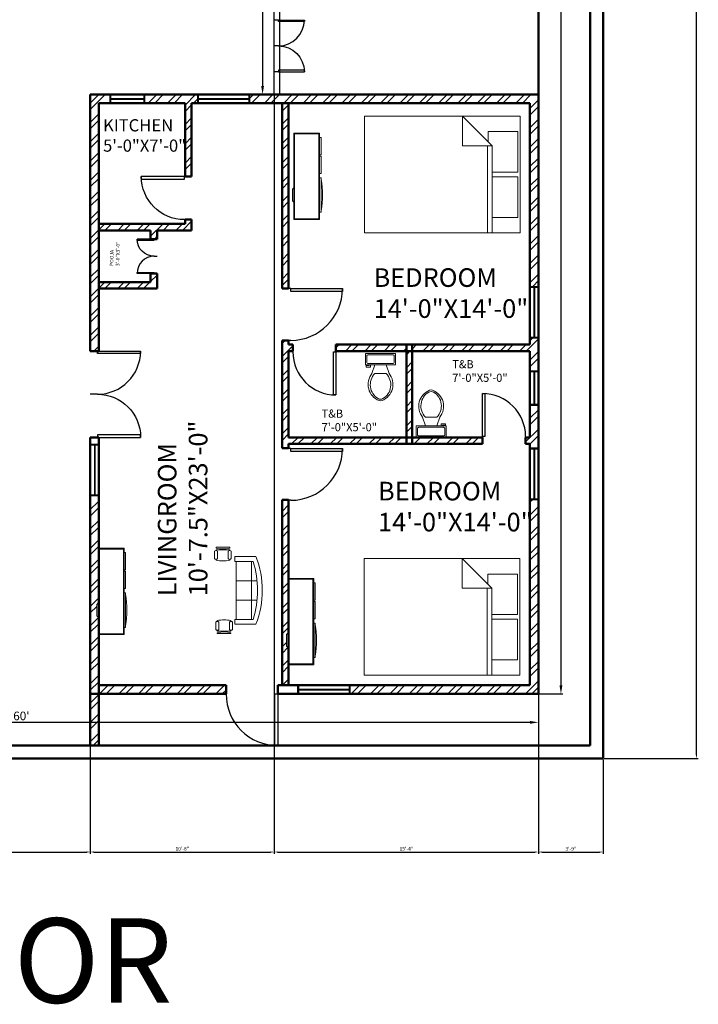
# Model space of a CAD drawing. Units: inches. Extents: x -12550 to 6516, y 1273 to 18700.
# Tile 13 of 19: x 4811 to 5284, y 1273 to 1958. Entities that reach past the tile are written whole.
import ezdxf

# ---------------------------------------------------------------- set-up
doc = ezdxf.new("R2010")
doc.units = ezdxf.units.IN
for name, color, linetype, lineweight in [('A-ANNO-DIMS', 2, 'Continuous', 18), ('A-ANNO-TEXT', 7, 'Continuous', 25), ('A-AREA-IDEN', 1, 'Continuous', 18), ('A-DOOR', 5, 'Continuous', 25), ('A-EQPM', 4, 'Continuous', 25), ('A-FURN', 8, 'Continuous', 18), ('A-GLAZ', 3, 'Continuous', 25), ('A-WALL', 7, 'Continuous', 50), ('A-WALL-PATT', 8, 'Continuous', 13)]:
    doc.layers.add(name, color=color, linetype=linetype, lineweight=lineweight)
doc.styles.get("Standard").update_dxf_attribs({"font": 'arial.ttf'})
doc.dimstyles.new('ISO-25', dxfattribs={"dimtxt": 2.5, "dimasz": 2.5, "dimexe": 1.25, "dimexo": 0.625, "dimtad": 1, "dimlunit": 4, "dimtxsty": 'Standard', "dimcen": 2.5, "dimadec": 0, "dimazin": 0, "dimtfac": 1, "dimtmove": 0, "dimatfit": 3, "dimfxl": 1, "dimarcsym": 0})
pattern_1 = [(45, (2434.941, 0), (-6.735192, 6.735192), []), (45, (2439.432, 0), (-6.735192, 6.735192), [])]

# ---------------------------------------------------------------- blocks, each defined once
blk = doc.blocks.new('*U2')
for p, q in [((0, 0), (0, -5)), ((30, 0), (30, -5))]:
    blk.add_line(p, q)
blk.add_lwpolyline([(0, 0), (0, 30), (1.75, 30), (1.75, 0)], close=True)
blk.add_arc((0, 0), 30, 0, 90)
blk = doc.blocks.new('Bed - Queen')
for p, q in [((0, -80.00003), (0, 0)), ((0, 0), (59.99999, 0)), ((59.99999, 0), (59.99999, -80.00003)), ((7.99999, -1.2), (28.79998, -1.2)), ((7.99999, -14.4), (7.99999, -1.2)), ((28.79998, -1.2), (28.79998, -14.4)), ((31.19999, -1.2), (51.99999, -1.2)), ((31.19999, -14.4), (31.19999, -1.2)), ((51.99999, -1.2), (51.99999, -16.4)), ((0, -14.4), (44.8, -14.4)), ((59.99999, -29.6), (44.8, -14.4)), ((44.8, -14.4), (44.8, -29.6)), ((44.8, -16.8), (0, -16.8)), ((51.99999, -16.4), (46.79936, -16.4)), ((44.8, -29.6), (59.99999, -29.6)), ((59.99999, -80.00003), (0, -80.00003))]:
    blk.add_line(p, q)
blk = doc.blocks.new('Toilet - top')
for p, q in [((9.5, -6), (9.5, -2)), ((-10, -8.5), (-8, -8.5)), ((-10, -9.5), (-10, -8.5)), ((-7, -9.5), (-10, -9.5)), ((-8, -8.5), (-8, -8)), ((-7, -8), (-7, -9.5)), ((-4, -8), (-6, -14)), ((4, -8), (6, -14)), ((4, -14), (-4, -14))]:
    blk.add_line(p, q)
blk.add_lwpolyline([(10.5, -8), (10.5, 0), (-10.5, 0), (-10.5, -8)], close=True)
for points in [[(-9.5, -2), (-9.5, -6)], [(8.5, -1), (-8.5, -1)], [(-8.5, -7), (8.5, -7)]]:
    blk.add_lwpolyline(points)
for centre, radius, start, end in [((-8.62, -1.88), 0.884, 81.8699, 188.1301), ((-8.62, -6.12), 0.884, 171.8699, 278.1301), ((8.62, -1.88), 0.884, 351.8699, 98.1301), ((8.62, -6.12), 0.884, 261.8699, 8.1301), ((3.52, -21.58), 12.17, 141.46911, 247.97143), ((4.2, -21.82), 11.33, 136.36773, 238.94682), ((-3.52, -21.58), 12.17, 292.02843, 38.53071), ((-4.2, -21.82), 11.33, 301.05301, 43.63209), ((0, -27.88), 4, 245.73182, 294.26817), ((0, -29), 4, 254.86053, 285.13947)]:
    blk.add_arc(centre, radius, start, end)
blk = doc.blocks.new('Entertainment Center')
for p, q in [((-4, 0), (-5, -1)), ((4, 0), (-4, 0)), ((5, -1), (4, 0)), ((-17, -19), (-17, -1)), ((-17, -1), (43, -1)), ((-16.5, -18.5), (-16.5, -1.5)), ((-16.5, -1.5), (42.5, -1.5)), ((42.5, -1.5), (42.5, -18.5)), ((43, -1), (43, -19)), ((43, -19), (-17, -19)), ((42.5, -18.5), (-16.5, -18.5)), ((-12, -20), (-12, -19)), ((12, -20), (-12, -20)), ((12, -19), (12, -20)), ((15, -20), (15, -19)), ((27, -20), (15, -20)), ((27, -19), (27, -20)), ((28, -20), (28, -19)), ((40, -20), (28, -20)), ((40, -19), (40, -20))]:
    blk.add_line(p, q)
blk.add_arc((0, 40), 61, 259.6111, 280.3889)
blk = doc.blocks.new('Sofa - Roundback 7 ft.')
for p, q in [((-36.000027, -34), (-36.000027, -11.4696)), ((-12.00002, -32.4421), (-12.00003, -6.5971)), ((11.99997, -32.4421), (11.99998, -6.5971)), ((35.99998, -34), (35.99998, -11.4696)), ((-35.999844, -13.3819), (35.9998, -13.3819)), ((-36.000027, -32.4421), (35.99998, -32.4421))]:
    blk.add_line(p, q)
for points in [[(-36.000027, -34), (-42.000027, -34), (-42.000027, -8)], [(41.99998, -8), (41.99998, -34), (35.99998, -34)]]:
    blk.add_lwpolyline(points)
for centre, radius, start, end in [((0, -114.25), 114.25, 68.43141, 111.5686), ((-0.00001, -127.1968), 121.1968, 72.72033, 107.2797)]:
    blk.add_arc(centre, radius, start, end)
blk = doc.blocks.new('Chair - Desk')
for p, q in [((-8.5, 0), (-8.5, -1)), ((-8.5, 0), (8.5, 0)), ((8.5, 0), (8.5, -1)), ((-10.5, -5), (-10.5, -14)), ((-8.5, -3), (-8.5, -4)), ((-8.5, -3), (8.5, -3)), ((-6.5, -14), (-6.5, -5)), ((-2, -3), (-2, -1.9355)), ((2, -1.9576), (2, -3)), ((6.5, -5), (6.5, -14)), ((8.5, -3), (8.5, -4)), ((10.5, -14), (10.5, -5)), ((-8.5, -15), (-8.5, -16)), ((8.5, -15), (8.5, -16))]:
    blk.add_line(p, q)
for centre, radius, start, end in [((-8.5, -6.5), 2.5, 36.8699, 143.1301), ((0, 34.625), 36.625, 256.5803, 283.4197), ((8.5, -6.5), 2.5, 36.8699, 143.1301), ((-8.5, -12.5), 2.5, 216.8699, 323.1301), ((0, 19.625), 36.625, 256.5803, 283.4197), ((8.5, -12.5), 2.5, 216.8699, 323.1301)]:
    blk.add_arc(centre, radius, start, end)
blk = doc.blocks.new('*D40')
at = {"layer": 'A-ANNO-DIMS', "color": 0, "lineweight": -2, "transparency": 16777216}
for p, q in [((4988.01, 2056.25), (4979.29, 2056.25)), ((4980.54, 2050.25), (4980.54, 1912.25)), ((4988.01, 1906.25), (4979.29, 1906.25))]:
    blk.add_line(p, q, dxfattribs=at)
at = {"layer": 'A-ANNO-DIMS', "color": 0, "transparency": 16777216}
for points in [[(4979.54, 2050.25), (4981.54, 2050.25), (4980.54, 2056.25)], [(4979.54, 1912.25), (4981.54, 1912.25), (4980.54, 1906.25)]]:
    blk.add_solid(points, dxfattribs=at)
at = {"layer": 'Defpoints', "color": 0, "transparency": 16777216}
for p in [(4988.63, 2056.25), (4980.54, 1906.25), (4988.63, 1906.25)]:
    blk.add_point(p, dxfattribs=at)
at = {"layer": 'A-ANNO-DIMS', "color": 0, "transparency": 16777216, "insert": (4976.86, 1981.25), "char_height": 6, "attachment_point": 5, "rotation": 90}
blk.add_mtext('12\'-6"', dxfattribs=at)
blk = doc.blocks.new('*D42')
at = {"layer": 'A-ANNO-DIMS', "color": 0, "lineweight": -2, "transparency": 16777216}
for p, q in [((5173.26, 2473.25), (5189.5, 2473.25)), ((5188.25, 2467.25), (5188.25, 1495.25)), ((5173.26, 1489.25), (5189.5, 1489.25))]:
    blk.add_line(p, q, dxfattribs=at)
at = {"layer": 'A-ANNO-DIMS', "color": 0, "transparency": 16777216}
for points in [[(5187.25, 2467.25), (5189.25, 2467.25), (5188.25, 2473.25)], [(5187.25, 1495.25), (5189.25, 1495.25), (5188.25, 1489.25)]]:
    blk.add_solid(points, dxfattribs=at)
at = {"layer": 'Defpoints', "color": 0, "transparency": 16777216}
for p in [(5172.63, 2473.25), (5172.63, 1489.25), (5188.25, 1489.25)]:
    blk.add_point(p, dxfattribs=at)
at = {"layer": 'A-ANNO-DIMS', "color": 0, "transparency": 16777216, "insert": (5184.56, 1981.25), "char_height": 6, "attachment_point": 5, "rotation": 90}
blk.add_mtext("82'", dxfattribs=at)
blk = doc.blocks.new('*D43')
at = {"layer": 'A-ANNO-DIMS', "color": 0, "lineweight": -2, "transparency": 16777216}
for p, q in [((4452.63, 1488.62), (4452.63, 1468.21)), ((5172.63, 1488.62), (5172.63, 1468.21)), ((5166.63, 1469.46), (4458.63, 1469.46))]:
    blk.add_line(p, q, dxfattribs=at)
at = {"layer": 'A-ANNO-DIMS', "color": 0, "transparency": 16777216}
for points in [[(4458.63, 1470.46), (4458.63, 1468.46), (4452.63, 1469.46)], [(5166.63, 1470.46), (5166.63, 1468.46), (5172.63, 1469.46)]]:
    blk.add_solid(points, dxfattribs=at)
at = {"layer": 'Defpoints', "color": 0, "transparency": 16777216}
for p in [(4452.63, 1489.25), (5172.63, 1489.25), (4452.63, 1469.46)]:
    blk.add_point(p, dxfattribs=at)
at = {"layer": 'A-ANNO-DIMS', "color": 0, "transparency": 16777216, "insert": (4812.63, 1473.15), "char_height": 6, "attachment_point": 5}
blk.add_mtext("60'", dxfattribs=at)
blk = doc.blocks.new('WIN-3FT')
for p, q in [((0, 0), (0, 6)), ((0, 6), (36.02, 6)), ((36.02, 0), (0, 0)), ((0.5, 0), (0.5, 6)), ((35.52, 3.2), (0.5, 3.2)), ((35.52, 2.8), (0.5, 2.8)), ((35.52, 6), (35.52, 0)), ((36.02, 6), (36.02, 0))]:
    blk.add_line(p, q)
blk = doc.blocks.new('WIN-2FT')
for p, q in [((0, 0), (0, 24.02)), ((0, 24.02), (6, 24.02)), ((0, 23.52), (6, 23.52)), ((2.8, 0.5), (2.8, 23.52)), ((3.2, 0.5), (3.2, 23.52)), ((6, 24.02), (6, 0)), ((6, 0.5), (0, 0.5)), ((6, 0), (0, 0))]:
    blk.add_line(p, q)
blk = doc.blocks.new('*D113')
at = {"layer": 'A-ANNO-DIMS', "color": 0, "lineweight": -2, "transparency": 16777216}
for p, q in [((5218.26, 2518.25), (5283.88, 2518.25)), ((5282.63, 1446.75), (5282.63, 2515.75)), ((5218.26, 1444.25), (5283.88, 1444.25))]:
    blk.add_line(p, q, dxfattribs=at)
at = {"layer": 'A-ANNO-DIMS', "color": 0, "transparency": 16777216}
for points in [[(5282.21, 2515.75), (5283.05, 2515.75), (5282.63, 2518.25)], [(5282.21, 1446.75), (5283.05, 1446.75), (5282.63, 1444.25)]]:
    blk.add_solid(points, dxfattribs=at)
at = {"layer": 'Defpoints', "color": 0, "transparency": 16777216}
for p in [(5217.63, 2518.25), (5282.63, 2518.25), (5217.63, 1444.25)]:
    blk.add_point(p, dxfattribs=at)
at = {"layer": 'A-ANNO-DIMS', "color": 0, "transparency": 16777216, "insert": (5280.73, 1981.25), "char_height": 2.5, "attachment_point": 5, "rotation": 90}
blk.add_mtext('89\'-6"', dxfattribs=at)
blk = doc.blocks.new('*D115')
at = {"layer": 'A-ANNO-DIMS', "color": 0, "lineweight": -2, "transparency": 16777216}
for p, q in [((4452.63, 1488.62), (4452.63, 1378)), ((4860.63, 1488.62), (4860.63, 1378)), ((4455.13, 1379.25), (4858.13, 1379.25))]:
    blk.add_line(p, q, dxfattribs=at)
at = {"layer": 'A-ANNO-DIMS', "color": 0, "transparency": 16777216}
for points in [[(4455.13, 1379.66), (4455.13, 1378.83), (4452.63, 1379.25)], [(4858.13, 1379.66), (4858.13, 1378.83), (4860.63, 1379.25)]]:
    blk.add_solid(points, dxfattribs=at)
at = {"layer": 'Defpoints', "color": 0, "transparency": 16777216}
for p in [(4452.63, 1489.25), (4860.63, 1489.25), (4860.63, 1379.25)]:
    blk.add_point(p, dxfattribs=at)
at = {"layer": 'A-ANNO-DIMS', "color": 0, "transparency": 16777216, "insert": (4656.63, 1381.15), "char_height": 2.5, "attachment_point": 5}
blk.add_mtext('34\'-0"', dxfattribs=at)
blk = doc.blocks.new('*D116')
at = {"layer": 'A-ANNO-DIMS', "color": 0, "lineweight": -2, "transparency": 16777216}
for p, q in [((4988.63, 1905.62), (4988.63, 1378)), ((4860.63, 1488.62), (4860.63, 1378)), ((4863.13, 1379.25), (4986.13, 1379.25))]:
    blk.add_line(p, q, dxfattribs=at)
at = {"layer": 'A-ANNO-DIMS', "color": 0, "transparency": 16777216}
for points in [[(4863.13, 1379.66), (4863.13, 1378.83), (4860.63, 1379.25)], [(4986.13, 1379.66), (4986.13, 1378.83), (4988.63, 1379.25)]]:
    blk.add_solid(points, dxfattribs=at)
at = {"layer": 'Defpoints', "color": 0, "transparency": 16777216}
for p in [(4988.63, 1906.25), (4860.63, 1489.25), (4988.63, 1379.25)]:
    blk.add_point(p, dxfattribs=at)
at = {"layer": 'A-ANNO-DIMS', "color": 0, "transparency": 16777216, "insert": (4924.63, 1381.15), "char_height": 2.5, "attachment_point": 5}
blk.add_mtext('10\'-8"', dxfattribs=at)
blk = doc.blocks.new('*D117')
at = {"layer": 'A-ANNO-DIMS', "color": 0, "lineweight": -2, "transparency": 16777216}
for p, q in [((4988.63, 1905.62), (4988.63, 1378)), ((5172.63, 1905.62), (5172.63, 1378)), ((4991.13, 1379.25), (5170.13, 1379.25))]:
    blk.add_line(p, q, dxfattribs=at)
at = {"layer": 'A-ANNO-DIMS', "color": 0, "transparency": 16777216}
for points in [[(4991.13, 1379.66), (4991.13, 1378.83), (4988.63, 1379.25)], [(5170.13, 1379.66), (5170.13, 1378.83), (5172.63, 1379.25)]]:
    blk.add_solid(points, dxfattribs=at)
at = {"layer": 'Defpoints', "color": 0, "transparency": 16777216}
for p in [(4988.63, 1906.25), (5172.63, 1906.25), (5172.63, 1379.25)]:
    blk.add_point(p, dxfattribs=at)
at = {"layer": 'A-ANNO-DIMS', "color": 0, "transparency": 16777216, "insert": (5080.63, 1381.15), "char_height": 2.5, "attachment_point": 5}
blk.add_mtext('15\'-4"', dxfattribs=at)
blk = doc.blocks.new('*D118')
at = {"layer": 'A-ANNO-DIMS', "color": 0, "lineweight": -2, "transparency": 16777216}
for p, q in [((5172.63, 1488.62), (5172.63, 1378)), ((5217.63, 1443.62), (5217.63, 1378)), ((5175.13, 1379.25), (5215.13, 1379.25))]:
    blk.add_line(p, q, dxfattribs=at)
at = {"layer": 'A-ANNO-DIMS', "color": 0, "transparency": 16777216}
for points in [[(5175.13, 1379.66), (5175.13, 1378.83), (5172.63, 1379.25)], [(5215.13, 1379.66), (5215.13, 1378.83), (5217.63, 1379.25)]]:
    blk.add_solid(points, dxfattribs=at)
at = {"layer": 'Defpoints', "color": 0, "transparency": 16777216}
for p in [(5172.63, 1489.25), (5217.63, 1444.25), (5217.63, 1379.25)]:
    blk.add_point(p, dxfattribs=at)
at = {"layer": 'A-ANNO-DIMS', "color": 0, "transparency": 16777216, "insert": (5195.13, 1381.15), "char_height": 2.5, "attachment_point": 5}
blk.add_mtext('3\'-9"', dxfattribs=at)

msp = doc.modelspace()

# ---------------------------------------------------------------- hatches: boundary and pattern name
at = {"layer": 'A-WALL-PATT'}
h = msp.add_hatch(dxfattribs=at)
h.set_pattern_fill('ANSI32', color=256)
h.set_pattern_definition(pattern_1)
h.paths.add_polyline_path([(4874.387, 1906.247), (4860.63, 1906.247), (4860.63, 1727.747), (4865.63, 1727.747), (4866.63, 1727.747), (4866.63, 1900.247), (4874.387, 1900.247)])
h = msp.add_hatch(dxfattribs=at)
h.set_pattern_fill('ANSI32', color=256)
h.set_pattern_definition(pattern_1)
h.paths.add_polyline_path([(4935.469, 1906.247), (4898.405, 1906.247), (4898.405, 1900.247), (4926.63, 1900.247), (4926.63, 1849.247), (4931.13, 1849.247), (4931.13, 1900.247), (4935.469, 1900.247)])
h = msp.add_hatch(dxfattribs=at)
h.set_pattern_fill('ANSI32', color=256)
h.set_pattern_definition(pattern_1)
h.paths.add_polyline_path([(5172.63, 1906.247), (4994.13, 1906.247), (4971.486, 1906.247), (4971.486, 1900.247), (4994.13, 1900.247), (5166.63, 1900.247), (5166.63, 1772.747), (5172.63, 1772.747)])
h = msp.add_hatch(dxfattribs=at)
h.set_pattern_fill('ANSI32', color=256)
h.set_pattern_definition(pattern_1)
h.paths.add_polyline_path([(4998.63, 1900.247), (4994.13, 1900.247), (4994.13, 1771.247), (4998.63, 1771.247)])
h = msp.add_hatch(dxfattribs=at)
h.set_pattern_fill('ANSI32', color=256)
h.set_pattern_definition(pattern_1)
h.paths.add_polyline_path([(4931.13, 1819.247), (4926.63, 1819.247), (4926.63, 1816.247), (4866.63, 1816.247), (4866.63, 1811.747), (4902.63, 1811.747), (4902.63, 1805.747), (4905.13, 1805.747), (4907.13, 1805.747), (4907.13, 1811.747), (4931.13, 1811.747)])
h = msp.add_hatch(dxfattribs=at)
h.set_pattern_fill('ANSI32', color=256)
h.set_pattern_definition(pattern_1)
h.paths.add_polyline_path([(4907.13, 1781.747), (4905.13, 1781.747), (4902.63, 1781.747), (4902.63, 1775.747), (4866.63, 1775.747), (4866.63, 1771.247), (4907.13, 1771.247)])
h = msp.add_hatch(dxfattribs=at)
h.set_pattern_fill('ANSI32', color=256)
h.set_pattern_definition(pattern_1)
h.paths.add_polyline_path([(4998.63, 1727.747), (5001.63, 1727.747), (5001.63, 1732.247), (4998.63, 1732.247), (4998.63, 1735.247), (4994.13, 1735.247), (4994.13, 1660.247), (4998.63, 1660.247), (4998.63, 1663.247), (5001.583, 1663.247), (5080.63, 1663.247), (5080.63, 1667.747), (5001.583, 1667.747), (4998.63, 1667.747)])
h = msp.add_hatch(dxfattribs=at)
h.set_pattern_fill('ANSI32', color=256)
h.set_pattern_definition(pattern_1)
h.paths.add_polyline_path([(5172.63, 1736.73), (5166.63, 1736.73), (5166.63, 1732.247), (5163.63, 1732.247), (5084.63, 1732.247), (5084.63, 1727.747), (5163.63, 1727.747), (5166.63, 1727.747), (5166.63, 1714.042), (5172.63, 1714.042)])
h = msp.add_hatch(dxfattribs=at)
h.set_pattern_fill('ANSI32', color=256)
h.set_pattern_definition(pattern_1)
h.paths.add_polyline_path([(5080.63, 1732.247), (5031.63, 1732.247), (5031.63, 1727.747), (5080.63, 1727.747)], flags=17)
h = msp.add_hatch(dxfattribs=at)
h.set_pattern_fill('ANSI32', color=256)
h.set_pattern_definition(pattern_1)
h.paths.add_polyline_path([(5084.63, 1727.747), (5080.63, 1727.747), (5080.63, 1667.747), (5084.63, 1667.747)])
h = msp.add_hatch(dxfattribs=at)
h.set_pattern_fill('ANSI32', color=256)
h.set_pattern_definition(pattern_1)
h.paths.add_polyline_path([(5172.63, 1690.024), (5166.63, 1690.024), (5166.63, 1667.747), (5163.63, 1667.747), (5163.63, 1663.247), (5166.63, 1663.247), (5166.63, 1660.369), (5172.63, 1660.369)])
h = msp.add_hatch(dxfattribs=at)
h.set_pattern_fill('ANSI32', color=256)
h.set_pattern_definition(pattern_1)
h.paths.add_polyline_path([(5133.63, 1667.747), (5084.63, 1667.747), (5084.63, 1663.247), (5133.63, 1663.247)])
h = msp.add_hatch(dxfattribs=at)
h.set_pattern_fill('ANSI32', color=256)
h.set_pattern_definition(pattern_1)
h.paths.add_polyline_path([(4955.13, 1495.247), (4866.63, 1495.247), (4866.63, 1530.559), (4866.13, 1530.559), (4866.13, 1542.559), (4865.13, 1543.559), (4865.13, 1551.559), (4866.13, 1552.559), (4866.13, 1590.559), (4866.366, 1627.032), (4860.63, 1627.032), (4860.63, 1489.247), (4955.13, 1489.247)])
h = msp.add_hatch(dxfattribs=at)
h.set_pattern_fill('ANSI32', color=256)
h.set_pattern_definition(pattern_1)
h.paths.add_polyline_path([(4994.13, 1623.947), (4994.13, 1495.247), (4998.63, 1495.247), (4998.63, 1509.575), (4998.13, 1509.575), (4998.13, 1521.575), (4997.13, 1522.575), (4997.13, 1530.575), (4998.13, 1531.575), (4998.13, 1569.575), (4998.627, 1623.947)])
h = msp.add_hatch(dxfattribs=at)
h.set_pattern_fill('ANSI32', color=256)
h.set_pattern_definition(pattern_1)
h.paths.add_polyline_path([(5172.63, 1624.352), (5166.63, 1624.352), (5166.63, 1495.247), (5041.216, 1495.247), (5041.216, 1489.247), (5172.63, 1489.247)])
h = msp.add_hatch(dxfattribs=at)
h.set_pattern_fill('ANSI32', color=256)
h.set_pattern_definition(pattern_1)
h.paths.add_polyline_path([(4866.63, 1489.247), (4860.63, 1489.247), (4860.63, 1453.247), (4866.63, 1453.247)])

# ---------------------------------------------------------------- linework, layer by layer
at = {"layer": 'A-EQPM'}
for p, q in [((4988.63, 1906.247), (4988.63, 2056.247)), ((4992.63, 1906.247), (4992.63, 2056.247)), ((5172.63, 2056.247), (5172.63, 1906.247)), ((5172.63, 1906.247), (4988.63, 1906.247))]:
    msp.add_line(p, q, dxfattribs=at)
at = {"layer": 'A-WALL'}
for p, q in [((5217.63, 2518.247), (5217.63, 1444.247)), ((5208.63, 2509.247), (5208.63, 1453.247)), ((5172.63, 1489.247), (5172.63, 2060.923)), ((5208.63, 1489.247), (5208.63, 2060.923)), ((4994.13, 1906.247), (4860.63, 1906.247)), ((4860.63, 1727.747), (4860.63, 1906.247)), ((5172.63, 1906.247), (4994.13, 1906.247)), ((4926.63, 1900.247), (4866.63, 1900.247)), ((4866.63, 1727.747), (4866.63, 1900.247)), ((4926.63, 1849.247), (4926.63, 1900.247)), ((4994.13, 1900.247), (4931.13, 1900.247)), ((4931.13, 1849.247), (4931.13, 1900.247)), ((5166.63, 1900.247), (4994.13, 1900.247)), ((4994.13, 1771.247), (4994.13, 1900.247)), ((4998.63, 1771.247), (4998.63, 1900.247)), ((5166.63, 1732.247), (5166.63, 1900.247)), ((4926.63, 1849.247), (4931.13, 1849.247)), ((4926.63, 1816.247), (4866.63, 1816.247)), ((4926.63, 1816.247), (4926.63, 1819.247)), ((4931.13, 1819.247), (4926.63, 1819.247)), ((4931.13, 1811.747), (4931.13, 1819.247)), ((4931.13, 1816.247), (4931.13, 1819.247)), ((4902.63, 1811.747), (4866.63, 1811.747)), ((4902.63, 1805.747), (4902.63, 1811.747)), ((4931.13, 1811.747), (4907.13, 1811.747)), ((4907.13, 1805.747), (4907.13, 1811.747)), ((4902.63, 1805.747), (4907.13, 1805.747)), ((4902.63, 1775.747), (4902.63, 1781.747)), ((4907.13, 1781.747), (4902.63, 1781.747)), ((4907.13, 1771.247), (4907.13, 1781.747)), ((4907.13, 1775.747), (4907.13, 1781.747)), ((4902.63, 1775.747), (4866.63, 1775.747)), ((4907.13, 1771.247), (4866.63, 1771.247)), ((4994.13, 1771.247), (4998.63, 1771.247)), ((4994.13, 1660.247), (4994.13, 1735.247)), ((4998.63, 1735.247), (4994.13, 1735.247)), ((4998.63, 1732.247), (4998.63, 1735.247)), ((4998.63, 1732.247), (4998.63, 1735.247)), ((4998.63, 1732.247), (4998.63, 1735.247)), ((4998.63, 1732.247), (4998.63, 1735.247)), ((4866.63, 1727.747), (4860.63, 1727.747)), ((5001.63, 1732.247), (4998.63, 1732.247)), ((5001.63, 1727.747), (4998.63, 1727.747)), ((4998.63, 1667.747), (4998.63, 1727.747)), ((4998.63, 1667.747), (4998.63, 1727.747)), ((4998.63, 1667.747), (4998.63, 1727.747)), ((4998.63, 1727.747), (5001.63, 1727.747)), ((5001.63, 1727.747), (5001.63, 1732.247)), ((5163.63, 1732.247), (5031.63, 1732.247)), ((5031.63, 1732.247), (5031.63, 1727.747)), ((5163.63, 1727.747), (5031.63, 1727.747)), ((5080.63, 1663.247), (5080.63, 1732.247)), ((5084.63, 1663.247), (5084.63, 1732.247)), ((5166.63, 1732.247), (5163.63, 1732.247)), ((5166.63, 1732.247), (5163.63, 1732.247)), ((5166.63, 1727.747), (5163.63, 1727.747)), ((5166.63, 1667.747), (5166.63, 1727.747)), ((4866.63, 1667.747), (4860.63, 1667.747)), ((4860.63, 1453.247), (4860.63, 1667.747)), ((4866.63, 1453.247), (4866.63, 1667.747)), ((5001.583, 1667.747), (4998.63, 1667.747)), ((5133.63, 1667.747), (5001.583, 1667.747)), ((5133.63, 1667.747), (5133.63, 1663.247)), ((5166.63, 1667.747), (5163.63, 1667.747)), ((5163.63, 1663.247), (5163.63, 1667.747)), ((4994.13, 1663.247), (4994.13, 1660.247)), ((4994.13, 1660.247), (4998.63, 1660.247)), ((5001.583, 1663.247), (4998.63, 1663.247)), ((4998.63, 1660.247), (4998.63, 1663.247)), ((4998.63, 1660.247), (4998.63, 1663.247)), ((4998.63, 1660.247), (4998.63, 1663.247)), ((5133.63, 1663.247), (5001.583, 1663.247)), ((5166.63, 1663.247), (5163.63, 1663.247)), ((5166.63, 1663.247), (5163.63, 1663.247)), ((5166.63, 1495.247), (5166.63, 1663.247)), ((4994.13, 1495.247), (4994.13, 1624.247)), ((4998.63, 1624.247), (4994.13, 1624.247)), ((4998.63, 1495.247), (4998.63, 1624.247)), ((4955.13, 1495.247), (4866.63, 1495.247)), ((4955.13, 1489.247), (4955.13, 1495.247)), ((5166.63, 1495.247), (4991.13, 1495.247)), ((4994.13, 1495.247), (4991.13, 1495.247)), ((4991.13, 1495.247), (4991.13, 1489.247)), ((4955.13, 1489.247), (4860.63, 1489.247)), ((5172.63, 1489.247), (4991.13, 1489.247)), ((4416.63, 1453.247), (5208.63, 1453.247)), ((4955.13, 1453.247), (4691.13, 1453.247)), ((4407.63, 1444.247), (5217.63, 1444.247))]:
    msp.add_line(p, q, dxfattribs=at)

# ---------------------------------------------------------------- block references
at = {"layer": 'A-DOOR', "xscale": -1}
for p, rotation in [((4926.13, 1849.247), 90), ((4865.63, 1667.747), 270)]:
    msp.add_blockref('*U2', p, dxfattribs=dict(at, rotation=rotation))
at = {"layer": 'A-DOOR'}
for p, xscale, yscale, zscale, rotation in [((4905.13, 1805.747), -0.399999999999997, 0.399999999999997, 0.399999999999997, 90), ((4905.13, 1781.747), 0.399999999999997, 0.399999999999997, 0.399999999999997, 90.00000000000003), ((5000.13, 1771.247), 1.199999999999999, 1.199999999999999, 1.199999999999999, 270), ((5000.13, 1659.947), 1.199999999999999, 1.199999999999999, 1.199999999999999, 270), ((4991.13, 1489.247), 1.199999999999999, 1.199999999999999, 1.199999999999999, 180)]:
    msp.add_blockref('*U2', p, dxfattribs=dict(at, xscale=xscale, yscale=yscale, zscale=zscale, rotation=rotation))
for p, rotation in [((4865.63, 1727.747), 270), ((5031.63, 1727.247), 180)]:
    msp.add_blockref('*U2', p, dxfattribs=dict(at, rotation=rotation))
msp.add_blockref('*U2', (5133.63, 1668.247), dxfattribs=at)
at = {"layer": 'A-EQPM', "yscale": 0.5999999999999954, "zscale": 0.5999999999999954, "rotation": 270}
for p, xscale in [((4991.63, 1958.135), 0.5999999999999954), ((4991.63, 1922.135), -0.5999999999999954)]:
    msp.add_blockref('*U2', p, dxfattribs=dict(at, xscale=xscale))
at = {"layer": 'A-FURN'}
for name, p, xscale, yscale, zscale, rotation in [('Bed - Queen', (5159.81, 1809.994), -1.354827908062564, 1.354827908062564, 1.354827908062564, 270), ('Sofa - Roundback 7 ft.', (4980.349, 1561.265), 0.5595223685495907, 0.5595223685495907, 0.5595223685495907, 270), ('Bed - Queen', (5159.649, 1502.217), -1.354827908062564, 1.354827908062564, 1.354827908062564, 270), ('Chair - Desk', (4953.764, 1531.281), 0.5595223685495907, 0.5595223685495907, 0.5595223685495907, 180)]:
    msp.add_blockref(name, p, dxfattribs=dict(at, xscale=xscale, yscale=yscale, zscale=zscale, rotation=rotation))
for name, p, rotation in [('Entertainment Center', (5001.26, 1836.379), 89.99999999999999), ('Toilet - top', (5097.899, 1667.747), 180), ('Entertainment Center', (4865.13, 1547.559), 89.99999999999999), ('Entertainment Center', (4997.13, 1526.575), 89.99999999999999)]:
    msp.add_blockref(name, p, dxfattribs=dict(at, rotation=rotation))
msp.add_blockref('Toilet - top', (5062.653, 1726.198), dxfattribs=at)
at = {"layer": 'A-FURN', "xscale": 0.5595223685495907, "yscale": 0.5595223685495907, "zscale": 0.5595223685495907}
msp.add_blockref('Chair - Desk', (4952.91, 1591.265), dxfattribs=at)
at = {"layer": 'A-GLAZ'}
for name, p, rotation in [('WIN-2FT', (4874.387, 1906.247), 269.9999999999974), ('WIN-3FT', (4971.486, 1906.247), 180), ('WIN-3FT', (5172.63, 1736.73), 90.0000000000048), ('WIN-2FT', (5172.63, 1714.042), 180), ('WIN-3FT', (4866.63, 1627.032), 90.000000000002), ('WIN-3FT', (5172.63, 1624.352), 90.00000000000468), ('WIN-3FT', (5041.216, 1495.247), 180)]:
    msp.add_blockref(name, p, dxfattribs=dict(at, rotation=rotation))

# ---------------------------------------------------------------- texts
at = {"layer": 'A-ANNO-TEXT', "insert": (4516.607, 1333.138), "char_height": 58.816, "attachment_point": 1}
msp.add_mtext('3rd FLOOR', dxfattribs=at)
at = {"layer": 'A-AREA-IDEN', "attachment_point": 1}
for s, width, gutter_width, insert, char_height in [('KITCHEN\\P5\'-0"X7\'-0"', 1.29487, 42.422, (4869.51, 1889.124), 8.48435), ('T&B\\P7\'-0"X5\'-0"', 4.19569, 28.328, (5112.552, 1721.465), 5.66556), ('T&B\\P7\'-0"X5\'-0"', 4.19569, 28.328, (5021.643, 1687.107), 5.66556)]:
    msp.add_mtext_dynamic_manual_height_columns(s, width=width, gutter_width=gutter_width, heights=[0], dxfattribs=dict(at, insert=insert, char_height=char_height))
at = {"layer": 'A-AREA-IDEN', "insert": (4874.182, 1787.026), "char_height": 2.5, "attachment_point": 1, "rotation": 89.183853}
msp.add_mtext_dynamic_manual_height_columns('POOJA\\P3\'-0"X3\'-0"', width=0.78585, gutter_width=12.5, heights=[0], dxfattribs=at)
at = {"layer": 'A-AREA-IDEN', "char_height": 12.93169, "attachment_point": 1}
for insert in [(5057.845, 1785.378), (5060.911, 1636.812)]:
    msp.add_mtext('BEDROOM\\P14\'-0"X14\'-0"', dxfattribs=dict(at, insert=insert))
at = {"layer": 'A-AREA-IDEN', "insert": (4907.654, 1557.153), "char_height": 12.93169, "attachment_point": 1, "rotation": 90}
msp.add_mtext('LIVINGROOM\\P10\'-7.5"X23\'-0"', dxfattribs=at)

# ---------------------------------------------------------------- dimensions: what is measured, and where the dimension line sits
at = {"layer": 'A-ANNO-DIMS'}
for base, p1, p2, override, picture, middle in [((5282.63, 2518.247), (5217.63, 1444.247), (5217.63, 2518.247), {"dimdec": 1, "dimlfac": 1, "dimrnd": 0, "dimzin": 1, "dimdsep": 46, "dimlunit": 4, "dimfrac": 2}, '*D113', (5280.729, 1981.247)), ((5188.25, 1489.247), (5172.63, 2473.247), (5172.63, 1489.247), {"dimtxt": 6, "dimasz": 6, "dimclrd": 0, "dimclre": 0, "dimclrt": 0}, '*D42', (5184.562, 1981.247)), ((4980.544, 1906.247), (4988.63, 2056.247), (4988.63, 1906.247), {"dimtxt": 6, "dimasz": 6, "dimclrd": 0, "dimclre": 0, "dimclrt": 0}, '*D40', (4976.855, 1981.247))]:
    dim = msp.add_linear_dim(base=base, p1=p1, p2=p2, angle=90, dimstyle='ISO-25', override=override, dxfattribs=at)
    dim.commit()
    dim.dimension.update_dxf_attribs({"geometry": picture, "text_midpoint": middle})
for base, p1, p2, override, picture, middle in [((4988.63, 1379.247), (4860.63, 1489.247), (4988.63, 1906.247), {"dimdec": 1, "dimlfac": 1, "dimrnd": 0, "dimzin": 1, "dimdsep": 46, "dimlunit": 4, "dimfrac": 2}, '*D116', (4924.63, 1381.149)), ((5172.63, 1379.247), (4988.63, 1906.247), (5172.63, 1906.247), {"dimdec": 1, "dimlfac": 1, "dimrnd": 0, "dimzin": 1, "dimdsep": 46, "dimlunit": 4, "dimfrac": 2}, '*D117', (5080.63, 1381.149)), ((4452.63, 1469.461), (5172.63, 1489.247), (4452.63, 1489.247), {"dimtxt": 6, "dimasz": 6, "dimclrd": 0, "dimclre": 0, "dimclrt": 0}, '*D43', (4812.63, 1473.15)), ((4860.63, 1379.247), (4452.63, 1489.247), (4860.63, 1489.247), {"dimdec": 1, "dimlfac": 1, "dimrnd": 0, "dimzin": 1, "dimdsep": 46, "dimlunit": 4, "dimfrac": 2}, '*D115', (4656.63, 1381.15)), ((5217.63, 1379.247), (5172.63, 1489.247), (5217.63, 1444.247), {"dimdec": 1, "dimlfac": 1, "dimrnd": 0, "dimzin": 1, "dimdsep": 46, "dimlunit": 4, "dimfrac": 2}, '*D118', (5195.13, 1381.15))]:
    dim = msp.add_linear_dim(base=base, p1=p1, p2=p2, dimstyle='ISO-25', override=override, dxfattribs=at)
    dim.commit()
    dim.dimension.update_dxf_attribs({"geometry": picture, "text_midpoint": middle})

doc.saveas('drawing.dxf')
